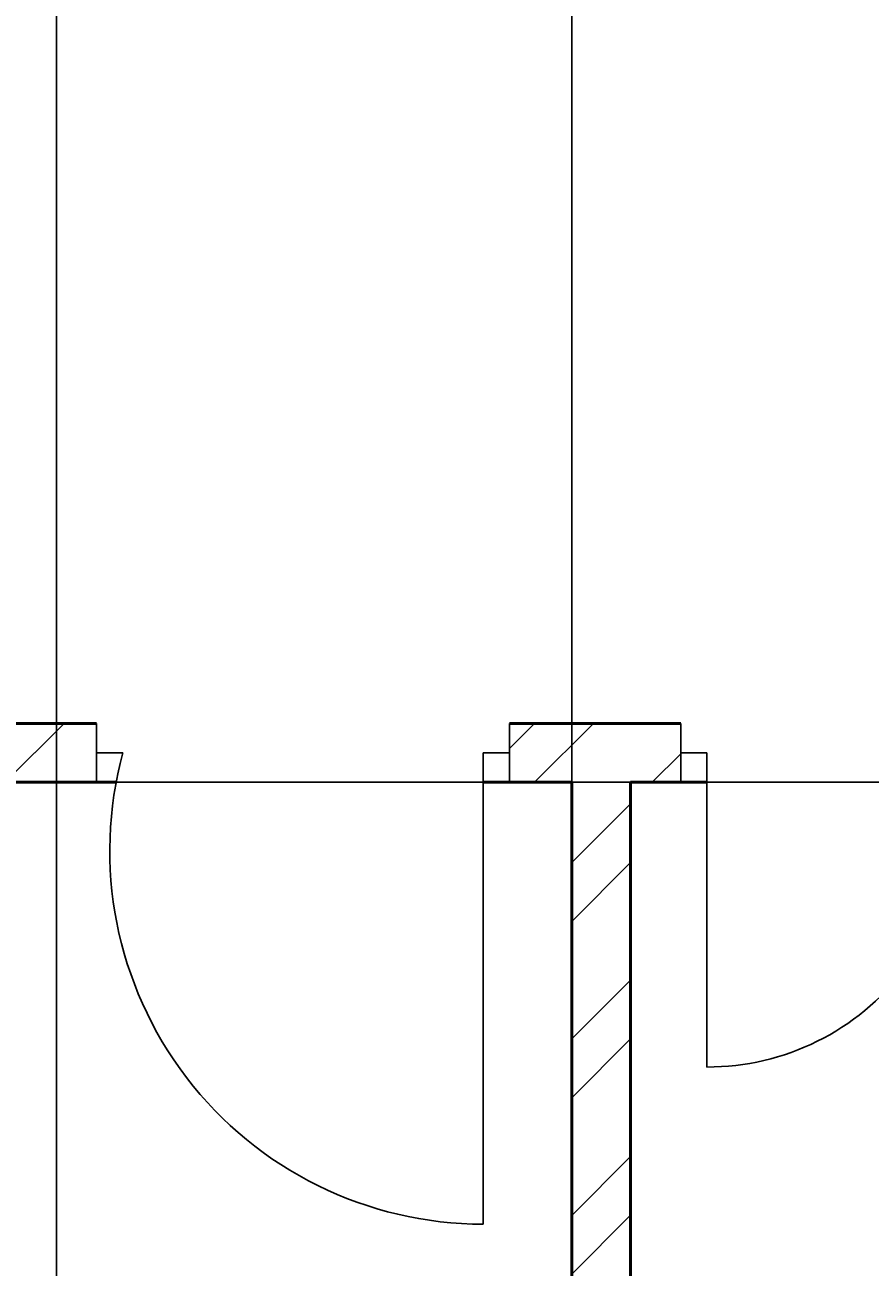
# Model space of a CAD drawing. Units: inches. Extents: x 2310 to 2937, y 1113 to 2410.
# Tile 12 of 23: x 2697 to 2761, y 1845 to 1940. Entities that reach past the tile are written whole.
import ezdxf

# ---------------------------------------------------------------- set-up
doc = ezdxf.new("R2010")
doc.units = ezdxf.units.IN
for name, color, linetype, lineweight in [('A-ANNO-DIMS', 2, 'Continuous', 18), ('A-DOOR', 31, 'Continuous', 25), ('A-WALL', 7, 'Continuous', 50), ('A-WALL-PATT', 85, 'Continuous', 13)]:
    doc.layers.add(name, color=color, linetype=linetype, lineweight=lineweight)
doc.styles.get("Standard").update_dxf_attribs({"font": 'arial.ttf'})
doc.dimstyles.get("Standard").update_dxf_attribs({"dimtxt": 0.18, "dimasz": 0.18, "dimexe": 0.18, "dimexo": 0.0625, "dimgap": 0.09, "dimtad": 0, "dimtih": 1, "dimtoh": 1, "dimdec": 4, "dimzin": 0, "dimdsep": 46, "dimtxsty": 'Standard', "dimcen": 0.09, "dimadec": 0, "dimazin": 0, "dimtfac": 1, "dimtdec": 4, "dimtofl": 0, "dimtmove": 0, "dimatfit": 3, "dimfxl": 1, "dimtolj": 1, "dimtzin": 0, "dimarcsym": 0})

# ---------------------------------------------------------------- blocks, each defined once
blk = doc.blocks.new('*D42')
at = {"layer": 'A-ANNO-DIMS', "color": 0, "lineweight": -2, "transparency": 16777216}
for p, q in [((2699.139, 2347.451), (2699.139, 1649.501)), ((2738.486, 2347.451), (2738.486, 1649.501)), ((2699.319, 1649.681), (2718.418, 1649.681)), ((2738.306, 1649.681), (2719.207, 1649.681))]:
    blk.add_line(p, q, dxfattribs=at)
at = {"layer": 'A-ANNO-DIMS', "color": 0, "transparency": 16777216}
for points in [[(2699.319, 1649.711), (2699.319, 1649.651), (2699.139, 1649.681)], [(2738.306, 1649.711), (2738.306, 1649.651), (2738.486, 1649.681)]]:
    blk.add_solid(points, dxfattribs=at)
at = {"layer": 'Defpoints', "color": 0, "transparency": 16777216}
for p in [(2699.139, 2347.514), (2738.486, 2347.514), (2738.486, 1649.681)]:
    blk.add_point(p, dxfattribs=at)
at = {"layer": 'A-ANNO-DIMS', "color": 0, "transparency": 16777216, "insert": (2718.813, 1649.681), "char_height": 0.18, "attachment_point": 5}
blk.add_mtext('\\A1;39.35', dxfattribs=at)
blk = doc.blocks.new('*D58')
at = {"layer": 'A-ANNO-DIMS', "color": 0, "lineweight": -2, "transparency": 16777216}
for p, q in [((2475.548, 1882.514), (2858.016, 1882.514)), ((2857.836, 1882.334), (2857.836, 1840.446)), ((2857.836, 1798.194), (2857.836, 1840.082)), ((2475.548, 1798.014), (2858.016, 1798.014))]:
    blk.add_line(p, q, dxfattribs=at)
at = {"layer": 'A-ANNO-DIMS', "color": 0, "transparency": 16777216}
for points in [[(2857.806, 1882.334), (2857.866, 1882.334), (2857.836, 1882.514)], [(2857.806, 1798.194), (2857.866, 1798.194), (2857.836, 1798.014)]]:
    blk.add_solid(points, dxfattribs=at)
at = {"layer": 'Defpoints', "color": 0, "transparency": 16777216}
for p in [(2475.486, 1882.514), (2857.836, 1882.514), (2475.486, 1798.014)]:
    blk.add_point(p, dxfattribs=at)
at = {"layer": 'A-ANNO-DIMS', "color": 0, "transparency": 16777216, "insert": (2857.836, 1840.264), "char_height": 0.18, "attachment_point": 5}
blk.add_mtext('\\A1;84.5', dxfattribs=at)

msp = doc.modelspace()

# ---------------------------------------------------------------- hatches: boundary and pattern name
at = {"layer": 'A-WALL-PATT'}
h = msp.add_hatch(dxfattribs=at)
h.set_pattern_fill('ANSI32', color=256)
h.paths.add_polyline_path([(2639.1394, 2356.5139), (2563.662, 2356.5139), (2563.662, 2347.5139), (2606.9859, 2347.5139), (2606.9859, 2210.5139), (2514.2692, 2210.5139), (2514.2692, 2206.0139), (2606.9859, 2206.0139), (2606.9859, 2098.0139), (2602.689, 2098.0139), (2602.689, 2093.5139), (2615.5262, 2093.5139), (2615.5262, 2095.7639), (2615.5262, 2098.0139), (2611.4859, 2098.0139), (2611.4859, 2206.0139), (2703.9391, 2206.0139), (2703.9391, 2208.2639), (2703.9391, 2210.5139), (2611.4859, 2210.5139), (2611.4859, 2347.5139), (2639.1394, 2347.5139)])
h.paths.add_polyline_path([(2823.9859, 2356.5139), (2699.1394, 2356.5139), (2699.1394, 2347.5139), (2738.4859, 2347.5139), (2738.4859, 2343.9266), (2742.9859, 2343.9266), (2742.9859, 2347.5139), (2814.9859, 2347.5139), (2814.9859, 2336.76), (2823.9859, 2336.76)])
h.paths.add_polyline_path([(2823.9859, 2312.76), (2814.9859, 2312.76), (2814.9859, 2299.5139), (2742.9859, 2299.5139), (2742.9859, 2323.0159), (2740.7359, 2323.0159), (2738.4859, 2323.0159), (2738.4859, 2210.5139), (2734.5483, 2210.5139), (2734.5483, 2206.0139), (2746.8769, 2206.0139), (2746.8769, 2208.2639), (2746.8769, 2210.5139), (2742.9859, 2210.5139), (2742.9859, 2295.0139), (2814.9859, 2295.0139), (2814.9859, 2269.8977), (2823.9859, 2269.8977)])
h.paths.add_polyline_path([(2823.9859, 2210.5139), (2823.9859, 2233.8977), (2819.4859, 2233.8977), (2814.9859, 2233.8977), (2814.9859, 2210.5139), (2769.9745, 2210.5139), (2769.9745, 2206.0139), (2814.9859, 2206.0139), (2814.9859, 2178.3027), (2823.9859, 2178.3027)])
h.paths.add_polyline_path([(2823.9859, 2118.3027), (2819.4859, 2118.3027), (2814.9859, 2118.3027), (2814.9859, 2098.0139), (2647.0333, 2098.0139), (2647.0333, 2093.5139), (2814.9859, 2093.5139), (2814.9859, 1999.5139), (2650.6052, 1999.5139), (2650.6052, 1995.0139), (2814.9859, 1995.0139), (2814.9859, 1969.9784), (2823.9859, 1969.9784)])
h.paths.add_polyline_path([(2403.4859, 2093.5139), (2569.9888, 2093.5139), (2569.9888, 2095.7639), (2569.9888, 2098.0139), (2403.4859, 2098.0139), (2403.4859, 2131.7587), (2394.4859, 2131.7587), (2394.4859, 1967.522), (2403.4859, 1967.522), (2403.4859, 1995.0139), (2569.8903, 1995.0139), (2569.8903, 1997.2639), (2569.8903, 1999.5139), (2403.4859, 1999.5139)])
h.paths.add_polyline_path([(2503.662, 2356.5139), (2394.4859, 2356.5139), (2394.4859, 2337.9231), (2398.9859, 2337.9231), (2403.4859, 2337.9231), (2403.4859, 2347.5139), (2475.4859, 2347.5139), (2475.4859, 2343.0384), (2479.9859, 2343.0384), (2479.9859, 2347.5139), (2503.662, 2347.5139)])
h.paths.add_polyline_path([(2498.3065, 1745.5139), (2479.9859, 1745.5139), (2479.9859, 1749.1663), (2477.7359, 1749.1663), (2475.4859, 1749.1663), (2475.4859, 1745.5139), (2403.4859, 1745.5139), (2403.4859, 1753.6409), (2398.9859, 1753.6409), (2394.4859, 1753.6409), (2394.4859, 1736.5139), (2498.3065, 1736.5139), (2498.3065, 1741.0139)])
h.paths.add_polyline_path([(2479.9859, 1882.5139), (2483.9367, 1882.5139), (2483.9367, 1887.0139), (2471.5501, 1887.0139), (2471.5501, 1885.1969), (2471.5501, 1882.5139), (2475.4859, 1882.5139), (2475.4859, 1798.0139), (2403.4859, 1798.0139), (2403.4859, 1828.0433), (2402.2852, 1828.0433), (2394.4859, 1828.0433), (2394.4859, 1777.6409), (2403.4859, 1777.6409), (2403.4859, 1793.5139), (2475.4859, 1793.5139), (2475.4859, 1769.1696), (2479.9859, 1769.1696)])
h.paths.add_polyline_path([(2403.4859, 1907.522), (2398.9859, 1907.522), (2394.4859, 1907.522), (2394.4859, 1864.0433), (2403.4859, 1864.0433), (2403.4859, 1882.5139), (2448.9325, 1882.5139), (2448.9325, 1884.7639), (2448.9325, 1887.0139), (2403.4859, 1887.0139)])
h.paths.add_polyline_path([(2702.2061, 1887.0139), (2611.4859, 1887.0139), (2611.4859, 1995.0139), (2615.6132, 1995.0139), (2615.6132, 1999.5139), (2602.4798, 1999.5139), (2602.4798, 1997.2639), (2602.4798, 1995.0139), (2606.9859, 1995.0139), (2606.9859, 1887.0139), (2516.2443, 1887.0139), (2516.2443, 1884.7639), (2516.2443, 1882.5139), (2606.9859, 1882.5139), (2606.9859, 1745.5139), (2558.3065, 1745.5139), (2558.3065, 1736.5139), (2638.8921, 1736.5139), (2638.8921, 1741.0139), (2638.8921, 1745.5139), (2611.4859, 1745.5139), (2611.4859, 1882.5139), (2702.2061, 1882.5139)])
h.paths.add_polyline_path([(2823.9859, 1909.9784), (2819.4859, 1909.9784), (2814.9859, 1909.9784), (2814.9859, 1887.0139), (2769.144, 1887.0139), (2769.144, 1884.7639), (2769.144, 1882.5139), (2814.9859, 1882.5139), (2814.9859, 1854.1704), (2823.9859, 1854.1704)])
h.paths.add_polyline_path([(2823.9859, 1818.1704), (2819.4859, 1818.1704), (2814.9859, 1818.1704), (2814.9859, 1798.0139), (2742.9859, 1798.0139), (2742.9859, 1882.5139), (2746.805, 1882.5139), (2746.805, 1887.0139), (2733.7334, 1887.0139), (2733.7334, 1884.7639), (2733.7334, 1882.5139), (2738.4859, 1882.5139), (2738.4859, 1771.1728), (2740.7359, 1771.1728), (2742.9859, 1771.1728), (2742.9859, 1793.5139), (2814.9859, 1793.5139), (2814.9859, 1783.6684), (2823.9859, 1783.6684)])
h.paths.add_polyline_path([(2823.9859, 1759.6684), (2814.9859, 1759.6684), (2814.9859, 1745.5139), (2742.9859, 1745.5139), (2742.9859, 1748.9831), (2740.7359, 1748.9831), (2738.4859, 1748.9831), (2738.4859, 1745.5139), (2698.8921, 1745.5139), (2698.8921, 1736.5139), (2823.9859, 1736.5139)])

# ---------------------------------------------------------------- linework, layer by layer
at = {"layer": 'A-DOOR'}
for p, q in [((2702.2061, 1882.5139), (2702.2061, 1887.0139)), ((2702.2061, 1887.0139), (2702.2061, 1884.7639)), ((2733.7334, 1882.5139), (2733.7334, 1887.0139)), ((2733.7334, 1887.0139), (2733.7334, 1884.7639)), ((2746.805, 1882.5139), (2746.805, 1887.0139)), ((2746.805, 1887.0139), (2746.805, 1884.7639)), ((2702.2061, 1884.7639), (2704.2061, 1884.7639)), ((2733.7334, 1884.7639), (2731.7334, 1884.7639)), ((2731.7334, 1884.7639), (2731.7334, 1848.7639)), ((2746.805, 1884.7639), (2748.805, 1884.7639)), ((2748.805, 1884.7639), (2748.805, 1860.7639))]:
    msp.add_line(p, q, dxfattribs=at)
for centre, radius, start, end in [((2731.7334, 1877.2883), 28.5243, 164.806485, 270), ((2748.805, 1879.7705), 19.0066, 270, 15.231482)]:
    msp.add_arc(centre, radius, start, end, dxfattribs=at)
at = {"layer": 'A-WALL'}
for p, q in [((2611.4859, 1887.0139), (2702.2061, 1887.0139)), ((2733.7334, 1887.0139), (2746.805, 1887.0139)), ((2611.4859, 1882.5139), (2703.6918, 1882.5139)), ((2731.7334, 1882.5139), (2738.4859, 1882.5139)), ((2738.4859, 1882.5139), (2738.4859, 1771.1728)), ((2742.9859, 1882.5139), (2742.9859, 1798.0139)), ((2742.9859, 1882.5139), (2748.805, 1882.5139))]:
    msp.add_line(p, q, dxfattribs=at)

# ---------------------------------------------------------------- dimensions: what is measured, and where the dimension line sits
at = {"layer": 'A-ANNO-DIMS'}
dim = msp.add_linear_dim(base=(2738.4859, 1649.6807), p1=(2699.1394, 2347.5139), p2=(2738.4859, 2347.5139), dimstyle='Standard', override={"dimdec": 2, "dimlfac": 1, "dimrnd": 0, "dimzin": 0, "dimdsep": 46, "dimlunit": 2}, dxfattribs=at)
dim.commit()
dim.dimension.update_dxf_attribs({"geometry": '*D42', "text_midpoint": (2718.8127, 1649.6807)})
dim = msp.add_linear_dim(base=(2857.8359, 1882.5139), p1=(2475.4859, 1798.0139), p2=(2475.4859, 1882.5139), angle=90, dimstyle='Standard', override={"dimdec": 1, "dimlfac": 1, "dimrnd": 0, "dimzin": 0, "dimdsep": 46, "dimlunit": 2}, dxfattribs=at)
dim.commit()
dim.dimension.update_dxf_attribs({"geometry": '*D58', "text_midpoint": (2857.8359, 1840.2639)})

doc.saveas('drawing.dxf')
